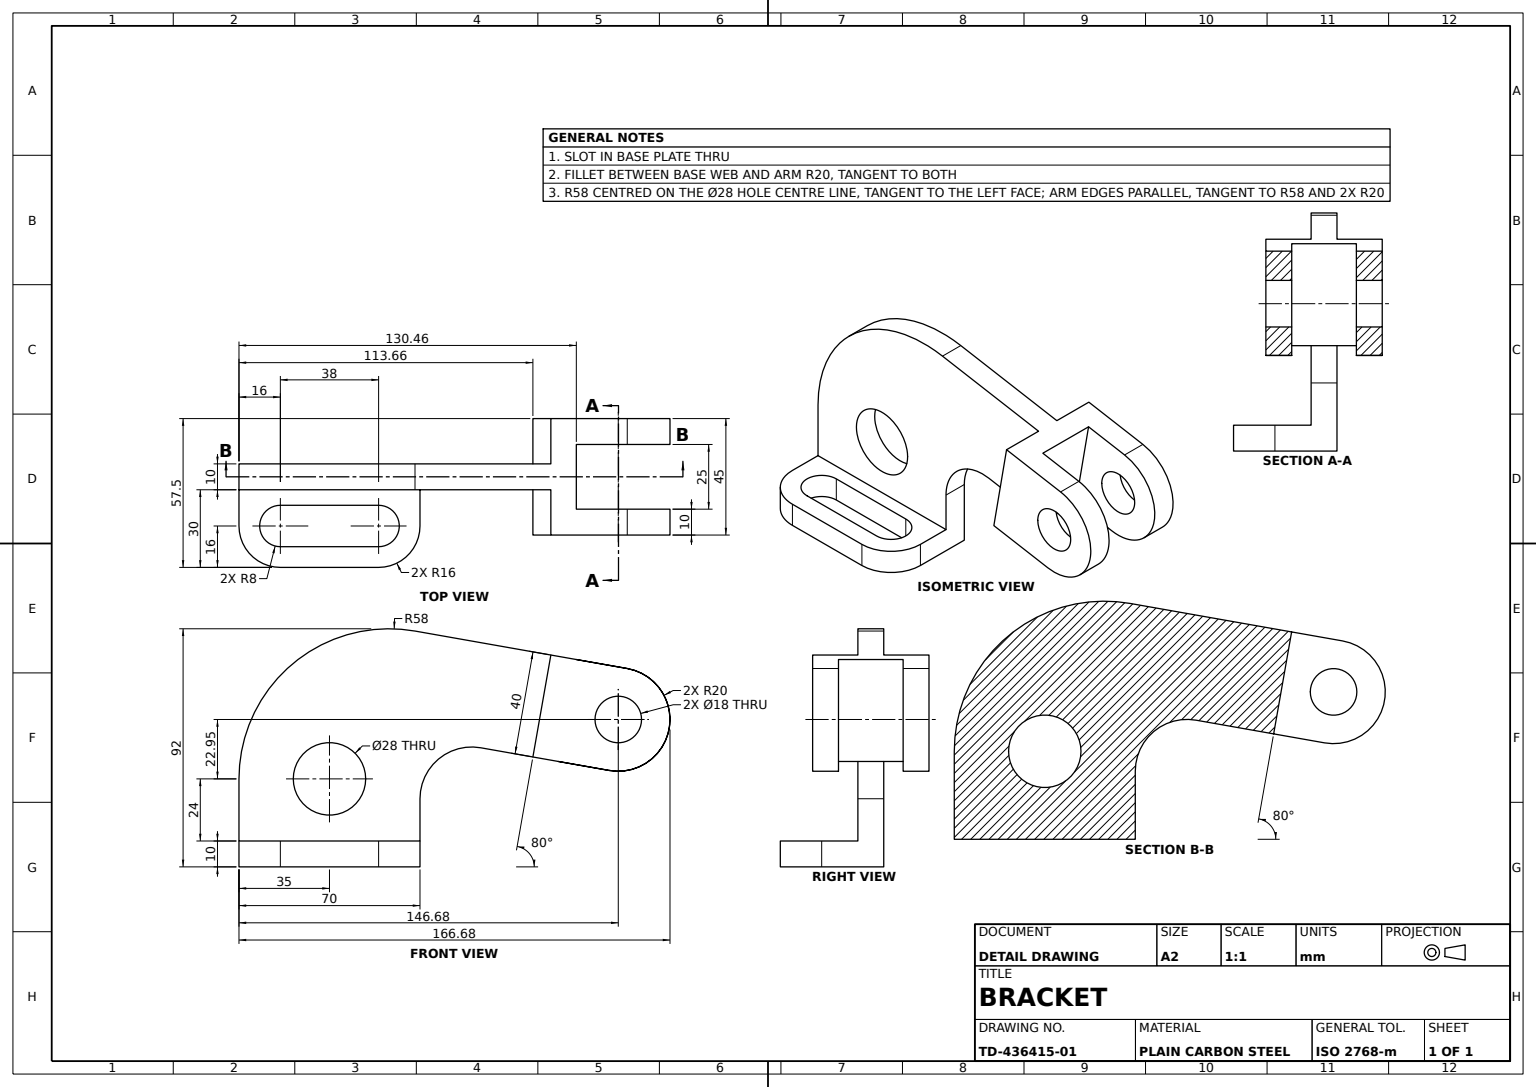
SolidWorks part; units mm, degrees
material "Plain Carbon Steel"
ref_plane "Front Plane" through (0, 0, 0) normal (0, 0, 1) x (1, 0, 0)
ref_plane "Top Plane" through (0, 0, 0) normal (0, 1, 0) x (1, 0, 0)
ref_plane "Right Plane" through (0, 0, 0) normal (1, 0, 0) x (0, 0, -1)
sketch "Base Plate Sketch" plane through (0, 0, 0) normal (0, 1, 0) x (1, 0, 0)
  line L0 (0, 0) -> (-70, 0)
  line L1 (-70, 0) -> (-70, -14)
  line L2 (-54, -30) -> (-16, -30)
  line L3 (0, -14) -> (0, 0)
  line L4 (-54, -14) -> (-16, -14) construction
  line L5 (-54, -6) -> (-16, -6)
  line L6 (-54, -22) -> (-16, -22)
  arc A0 (-16, -30) -> (0, -14) centre (-16, -14) ccw
  arc A1 (-70, -14) -> (-54, -30) centre (-54, -14) ccw
  arc A2 (-54, -6) -> (-54, -22) centre (-54, -14) ccw
  arc A3 (-16, -22) -> (-16, -6) centre (-16, -14) ccw
  point P3 (-35, -14)
  point P10 (-70, -30)
  dimension "D2" = 16
  dimension "D1" = 30
  dimension "D3" = 70
  dimension "D4" = 16
extrude "Slotted Base Plate" add sketch "Base Plate Sketch" along normal blind 10
sketch "Upright Web Sketch" plane through (0, 0, 0) normal (0, 0, -1) x (-1, 0, 0)
  line L0 (70, 0) -> (70, 34)
  line L1 (0, 0) -> (0, 26.3267)
  line L3 (70, 0) -> (0, 0)
  line L5 (70, 34) -> (70, 103.1217) construction
  line L6 (70, 103.1217) -> (1.9284, 91.1188) construction
  line L7 (1.9284, 91.1188) -> (-50.6105, 81.8548)
  line L8 (54, 10) -> (16, 10) construction
  line L9 (-23.473, 46.0228) -> (-43.6646, 42.4625)
  line L10 (-50.6105, 81.8548) -> (-43.6646, 42.4625)
  circle A0 centre (35, 34) radius 14
  arc A2 (70, 34) -> (1.9284, 91.1188) centre (12, 34) ccw
  arc A3 (0, 26.3267) -> (-23.473, 46.0228) centre (-20, 26.3267) ccw
  dimension "D2" = 28
  dimension "D3" = 80
  dimension "D4" = 58
  dimension "D6" = 20
  dimension "D1" = 24
  dimension "D5" = 40
  dimension "D7" = 35
  dimension "D8" = 76
extrude "Upright Web" add sketch "Upright Web Sketch" along normal blind 10
sketch "Clevis Arm Sketch" plane through (15.5241, 88.0415, 0) normal (0.1736, 0.9848, 0) x (0.9848, -0.1736, 0)
  line L0 (-17.7217, 10) -> (-17.7217, 0) construction
  line L1 (35.6277, 27.5) -> (45.6277, 27.5)
  line L2 (35.6277, 27.5) -> (35.6277, -17.5)
  line L4 (45.6277, 17.5) -> (45.6277, -7.5)
  line L5 (45.6277, 27.5) -> (65.6277, 27.5)
  line L7 (45.6277, 17.5) -> (65.6277, 17.5)
  line L8 (65.6277, 27.5) -> (65.6277, 17.5)
  line L9 (35.6277, -17.5) -> (65.6277, -17.5)
  line L11 (45.6277, -7.5) -> (65.6277, -7.5)
  line L12 (65.6277, -17.5) -> (65.6277, -7.5)
  point P10 (35.6277, 5)
  point P13 (-17.7217, 5)
  point P14 (45.6277, 5)
  dimension "D1" = 10
  dimension "D2" = 30
  dimension "D3" = 45
  dimension "D4" = 25
  dimension "D5" = 35.6277
extrude "Clevis Arm" add sketch "Clevis Arm Sketch" against normal blind 40
sketch "Clevis Ear 1 Sketch" plane through (0, 0, 17.5) normal (0, 0, 1) x (1, 0, 0)
  line L0 (73.2088, 37.2531) -> (80.1548, 76.6454) construction
  circle A0 centre (76.6818, 56.9492) radius 20
  dimension "D1" = 40
extrude "Clevis Ear 1" add sketch "Clevis Ear 1 Sketch" against normal up to surface (10 mm away) up to face at (66.8337, 58.6857, 7.5)
sketch "Clevis Ear 2 Sketch" plane through (0, 0, -27.5) normal (0, 0, -1) x (-1, 0, 0)
  circle A1 centre (-76.6818, 56.9492) radius 20
  circle A2 centre (-76.6818, 56.9492) radius 20
  dimension "D1" = 0
extrude "Clevis Ear 2" add sketch "Clevis Ear 2 Sketch" against normal up to surface (10 mm away) up to face at (66.8337, 58.6857, -17.5)
sketch "Clevis Pin Hole Sketch" plane through (0, 0, 17.5) normal (0, 0, 1) x (1, 0, 0)
  circle A0 centre (76.6818, 56.9492) radius 9
  arc A1 (73.2088, 37.2531) -> (80.1548, 76.6454) centre (76.6818, 56.9492) ccw construction
  dimension "D1" = 18
extrude "Clevis Pin Hole Ø18" cut sketch "Clevis Pin Hole Sketch" against normal through all
